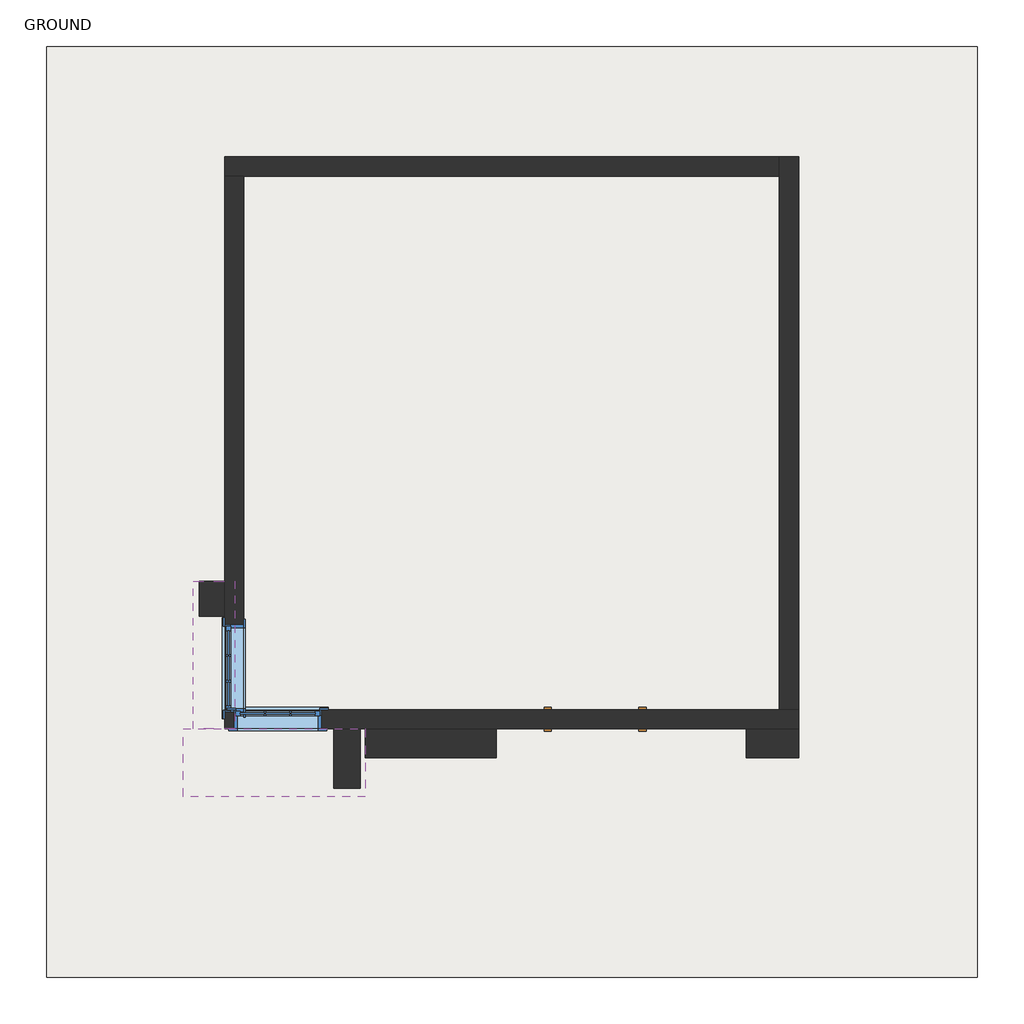
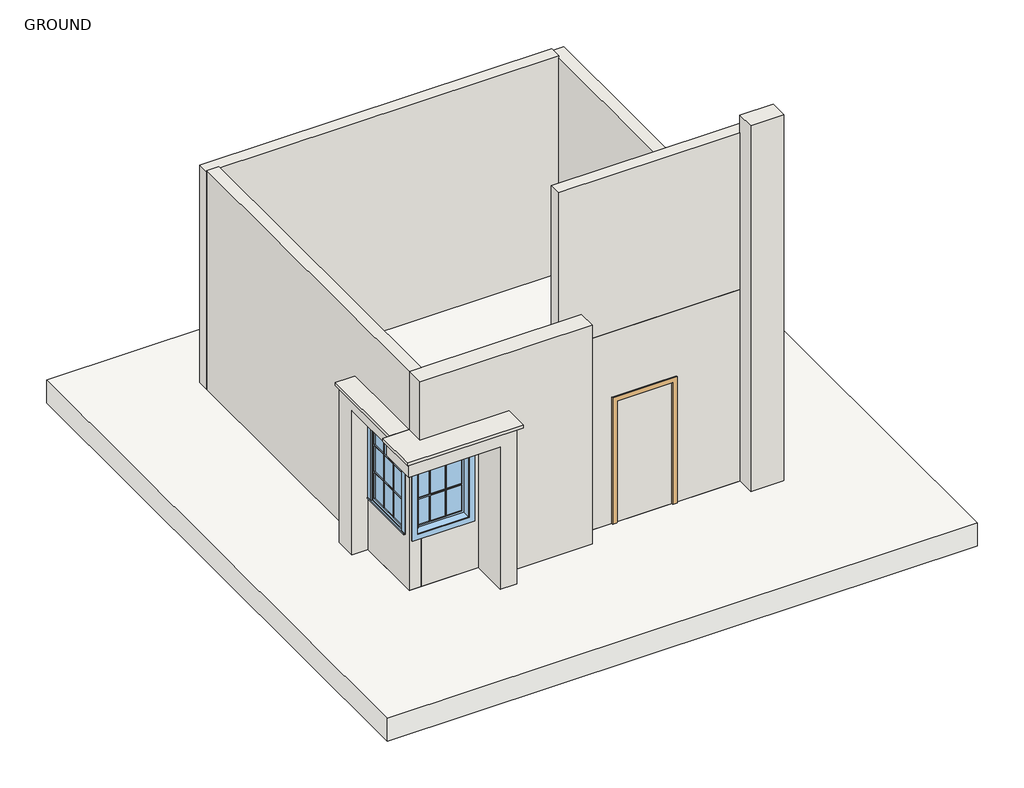
# One storey: 11 walls, 2 slabs, 2 windows, 1 door.
"""IFC4 building model written with IfcOpenShell, lengths in millimetres."""

from ifc_helpers import new_model, si_unit, frame, origin, place, context, project, spatial, polyline, outline, extrude, faceted_brep, transform, mapped, element, save
from components import m_single_flush_0915_x_2134mm_6a9e8738, walls_1_walls_1_8bdf3cb7, walls_10_walls_10_64d1ab67, walls_2_walls_2_b5bda089, walls_3_walls_3_8b246382, walls_5_walls_5_8fe41d8f, walls_6_walls_6_d361cd03, walls_9_walls_9_f00b2fad, window_3d3a5413

model = new_model("IFC4")

# Units and contexts
model_context = context("Model", 3, world=origin())
ifc_project = project(units=[si_unit("LENGTHUNIT", "METRE", prefix="MILLI")], contexts=[model_context])

# Site, building, storey
site = spatial("IfcSite", under=ifc_project)
building = spatial("IfcBuilding", under=site)
storey = spatial("IfcBuildingStorey", under=building, Name="GROUND", Elevation=0.0)

# Door
placement = place(None, origin())
m_single_flush_0915_x_2134mm_shape = m_single_flush_0915_x_2134mm_6a9e8738(model_context)
element("IfcDoor", 1, ObjectType="M_Single-Flush : 0915 x 2134mm", at=placement, inside=storey, context=model_context, shape_type="MappedRepresentation", body=[
    mapped(m_single_flush_0915_x_2134mm_shape, transform((-11916.6283679, -3290.9180898, 0.0), x_axis=(-1.0, 0.0, 0.0), y_axis=(0.0, -1.0, 0.0), z_axis=(0.0, 0.0, 1.0))),
])

# Slabs
element("IfcSlab", 2, ObjectType="Generic Floor - 400mm", at=placement, inside=storey, context=model_context, shape_type="SweptSolid", body=[
    extrude(outline(polyline([(-9784.4289001, -3390.9180898), (-15798.6897324, -3390.9180898), (-15798.6897324, 2600.2819102), (-9784.4289001, 2600.2819102), (-9784.4289001, -3390.9180898)])), frame((0.0, 0.0, -400.0), z_axis=(0.0, 0.0, 1.0), x_axis=(1.0, 0.0, 0.0)), (0.0, 0.0, 1.0), 400.0),
])
element("IfcSlab", 3, ObjectType="Generic Floor - 400mm", at=placement, inside=storey, context=model_context, shape_type="SweptSolid", body=[
    extrude(outline(polyline([(-7910.3714198, 3757.0368614), (-7910.3714198, -5996.5631386), (-17663.9714198, -5996.5631386), (-17663.9714198, 3757.0368614), (-7910.3714198, 3757.0368614)])), frame((0.0, 0.0, -400.0), z_axis=(0.0, 0.0, 1.0), x_axis=(1.0, 0.0, 0.0)), (0.0, 0.0, 1.0), 400.0),
])

# Walls
element("IfcWall", 4, ObjectType="Generic - 9\"", at=placement, inside=storey, context=model_context, shape_type="Brep", body=[
    faceted_brep([(-15798.6897324, 2400.2819102, 0.0), (-15598.6897324, 2400.2819102, 0.0), (-9984.4289001, 2400.2819102, 0.0), (-9984.4289001, 2400.2819102, 3805.8986036), (-15798.6897324, 2400.2819102, 3805.8986036), (-15798.6897324, 2600.2819102, 0.0), (-15798.6897324, 2600.2819102, 3805.8986036), (-9984.4289001, 2600.2819102, 3805.8986036), (-9984.4289001, 2600.2819102, 3774.1343037), (-9984.4289001, 2600.2819102, 0.0)], [[[0, 1, 2, 3, 4]], [[5, 6, 7, 8, 9]], [[2, 1, 0, 5, 9]], [[4, 3, 7, 6]], [[0, 4, 6, 5]], [[3, 2, 9, 8, 7]]]),
])
element("IfcWall", 5, ObjectType="Generic - 9\"", at=placement, inside=storey, context=model_context, shape_type="Brep", body=[
    faceted_brep([(-15598.6897324, -3390.9180898, 0.0), (-15598.6897324, -3190.9180898, 0.0), (-15598.6897324, 2400.2819102, 0.0), (-15598.6897324, 2400.2819102, 3830.5245478), (-15598.6897324, -3390.9180898, 3830.5245478), (-15598.6897324, -3390.9180898, 3352.8), (-15598.6897324, -3390.9180898, 2438.4), (-15598.6897324, -3190.9180898, 2438.4), (-15598.6897324, -2300.3180898, 2438.4), (-15598.6897324, -2300.3180898, 914.4), (-15598.6897324, -3190.9180898, 914.4), (-15598.6897324, -3390.9180898, 914.4), (-15798.6897324, 2400.2819102, 0.0), (-15798.6897324, -3390.9180898, 0.0), (-15798.6897324, -3390.9180898, 3830.5245478), (-15798.6897324, 2400.2819102, 3830.5245478), (-15798.6897324, 2400.2819102, 3805.8986036), (-15798.6897324, -2300.3180898, 914.4), (-15798.6897324, -2300.3180898, 2438.4), (-15798.6897324, -3214.7180898, 2438.4), (-15798.6897324, -3214.7180898, 914.4), (-15698.6897324, -3390.9180898, 914.4), (-15698.6897324, -3390.9180898, 2438.4), (-15698.6897324, -3214.7180898, 914.4), (-15698.6897324, -3214.7180898, 2438.4)], [[[0, 1, 2, 3, 4, 5, 6, 7, 8, 9, 10, 11]], [[12, 13, 14, 15, 16], [17, 18, 19, 20]], [[2, 1, 0, 13, 12]], [[4, 3, 15, 14]], [[4, 14, 13, 0, 11, 21, 22, 6, 5]], [[3, 2, 12, 16, 15]], [[9, 8, 18, 17]], [[17, 20, 23, 21, 11, 10, 9]], [[20, 19, 24, 23]], [[19, 18, 8, 7, 6, 22, 24]], [[21, 23, 24, 22]]]),
])
element("IfcWall", 6, ObjectType="Generic - 9\"", at=placement, inside=storey, context=model_context, shape_type="Brep", body=[
    faceted_brep([(-9784.4289001, -3190.9180898, 0.0), (-9984.4289001, -3190.9180898, 0.0), (-15598.6897324, -3190.9180898, 0.0), (-15598.6897324, -3190.9180898, 914.4), (-14784.2897324, -3190.9180898, 914.4), (-14784.2897324, -3190.9180898, 2438.4), (-15598.6897324, -3190.9180898, 2438.4), (-15598.6897324, -3190.9180898, 3352.8), (-9984.4289001, -3190.9180898, 3352.8), (-9784.4289001, -3190.9180898, 3352.8), (-15598.6897324, -3390.9180898, 0.0), (-9784.4289001, -3390.9180898, 0.0), (-9784.4289001, -3390.9180898, 3352.8), (-9984.4289001, -3390.9180898, 3352.8), (-15598.6897324, -3390.9180898, 3352.8), (-15598.6897324, -3390.9180898, 2438.4), (-14784.2897324, -3390.9180898, 2438.4), (-14784.2897324, -3390.9180898, 914.4), (-15598.6897324, -3390.9180898, 914.4)], [[[0, 1, 2, 3, 4, 5, 6, 7, 8, 9]], [[10, 11, 12, 13, 14, 15, 16, 17, 18]], [[2, 1, 0, 11, 10]], [[9, 8, 7, 14, 13, 12]], [[14, 7, 6, 15]], [[2, 10, 18, 3]], [[16, 5, 4, 17]], [[17, 4, 3, 18]], [[5, 16, 15, 6]], [[9, 12, 11, 0]]]),
])
element("IfcWall", 7, ObjectType="Generic - 9\"", at=placement, inside=storey, context=model_context, shape_type="Brep", body=[
    faceted_brep([(-9984.4289001, 2600.2819102, 0.0), (-9984.4289001, 2400.2819102, 0.0), (-9984.4289001, -3190.9180898, 0.0), (-9984.4289001, -3190.9180898, 3352.8), (-9984.4289001, -3390.9180898, 3352.8), (-9984.4289001, -3390.9180898, 3774.1343037), (-9984.4289001, -3190.9180898, 3774.1343037), (-9984.4289001, 2600.2819102, 3774.1343037), (-9784.4289001, 2600.2819102, 0.0), (-9784.4289001, 2600.2819102, 3774.1343037), (-9784.4289001, -3190.9180898, 3774.1343037), (-9784.4289001, -3390.9180898, 3774.1343037), (-9784.4289001, -3390.9180898, 3352.8), (-9784.4289001, -3190.9180898, 3352.8), (-9784.4289001, -3190.9180898, 0.0)], [[[0, 1, 2, 3, 4, 5, 6, 7]], [[8, 9, 10, 11, 12, 13, 14]], [[2, 1, 0, 8, 14]], [[7, 6, 5, 11, 10, 9]], [[0, 7, 9, 8]], [[12, 4, 3, 13]], [[2, 14, 13, 3]], [[5, 4, 12, 11]]]),
])
walls_1_walls_1_shape = walls_1_walls_1_8bdf3cb7(model_context)
element("IfcWall", 8, ObjectType="Walls 1 : Walls 1", at=placement, inside=storey, context=model_context, shape_type="MappedRepresentation", body=[
    mapped(walls_1_walls_1_shape, transform((0.0, 0.0, 0.0), x_axis=(1.0, 0.0, 0.0), y_axis=(0.0, 1.0, 0.0), z_axis=(0.0, 0.0, 1.0))),
])
walls_10_walls_10_shape = walls_10_walls_10_64d1ab67(model_context)
element("IfcWall", 9, ObjectType="Walls 10 : Walls 10", at=placement, inside=storey, context=model_context, shape_type="MappedRepresentation", body=[
    mapped(walls_10_walls_10_shape, transform((0.0, 0.0, 0.0), x_axis=(1.0, 0.0, 0.0), y_axis=(0.0, 1.0, 0.0), z_axis=(0.0, 0.0, 1.0))),
])
walls_2_walls_2_shape = walls_2_walls_2_b5bda089(model_context)
element("IfcWall", 10, ObjectType="Walls 2 : Walls 2", at=placement, inside=storey, context=model_context, shape_type="MappedRepresentation", body=[
    mapped(walls_2_walls_2_shape, transform((0.0, 0.0, 0.0), x_axis=(1.0, 0.0, 0.0), y_axis=(0.0, 1.0, 0.0), z_axis=(0.0, 0.0, 1.0))),
])
walls_3_walls_3_shape = walls_3_walls_3_8b246382(model_context)
element("IfcWall", 11, ObjectType="Walls 3 : Walls 3", at=placement, inside=storey, context=model_context, shape_type="MappedRepresentation", body=[
    mapped(walls_3_walls_3_shape, transform((0.0, 0.0, 0.0), x_axis=(1.0, 0.0, 0.0), y_axis=(0.0, 1.0, 0.0), z_axis=(0.0, 0.0, 1.0))),
])
walls_5_walls_5_shape = walls_5_walls_5_8fe41d8f(model_context)
element("IfcWall", 12, ObjectType="Walls 5 : Walls 5", at=placement, inside=storey, context=model_context, shape_type="MappedRepresentation", body=[
    mapped(walls_5_walls_5_shape, transform((0.0, 0.0, 0.0), x_axis=(1.0, 0.0, 0.0), y_axis=(0.0, 1.0, 0.0), z_axis=(0.0, 0.0, 1.0))),
])
walls_6_walls_6_shape = walls_6_walls_6_d361cd03(model_context)
element("IfcWall", 13, ObjectType="Walls 6 : Walls 6", at=placement, inside=storey, context=model_context, shape_type="MappedRepresentation", body=[
    mapped(walls_6_walls_6_shape, transform((0.0, 0.0, 0.0), x_axis=(1.0, 0.0, 0.0), y_axis=(0.0, 1.0, 0.0), z_axis=(0.0, 0.0, 1.0))),
])
walls_9_walls_9_shape = walls_9_walls_9_f00b2fad(model_context)
element("IfcWall", 14, ObjectType="Walls 9 : Walls 9", at=placement, inside=storey, context=model_context, shape_type="MappedRepresentation", body=[
    mapped(walls_9_walls_9_shape, transform((0.0, 0.0, 0.0), x_axis=(1.0, 0.0, 0.0), y_axis=(0.0, 1.0, 0.0), z_axis=(0.0, 0.0, 1.0))),
])

# Windows
window_shape = window_3d3a5413(model_context)
element("IfcWindow", 15, ObjectType="Casement 3x3 with Trim : 36\" x 60\"", at=placement, inside=storey, context=model_context, shape_type="MappedRepresentation", body=[
    mapped(window_shape, transform((-15241.4897324, -3290.9180898, 304.8), x_axis=(1.0, 0.0, 0.0), y_axis=(0.0, 1.0, 0.0), z_axis=(0.0, 0.0, 1.0))),
])
element("IfcWindow", 16, ObjectType="Casement 3x3 with Trim : 36\" x 60\"", at=placement, inside=storey, context=model_context, shape_type="MappedRepresentation", body=[
    mapped(window_shape, transform((-15698.6897324, -2757.5180898, 304.8), x_axis=(0.0, 1.0, 0.0), y_axis=(-1.0, 0.0, 0.0), z_axis=(0.0, 0.0, 1.0))),
])

save(model, "model.ifc")

# Revit data of these elements
# Type "M_Single-Flush : 0915 x 2134mm"
#   Type Mark = "15"
#   Thickness = 0' - 2.00787"
#   Height = 7' - 0.01575"
#   Trim Projection Ext = 0' - 0.98425"
#   Trim Projection Int = 0' - 0.98425"
#   Trim Width = 0' - 2.99213"
#   Width = 3' - 0.02362"
#   Door Material = Door - Panel
#   Frame Material = Door - Frame
#   Function = (empty or 0)
#   Wall Closure = (empty or 0)
# Type "Generic Floor - 400mm"
#   Function = 0
#   Layers, outside or top first: 1' - 3.74803" no material (function 1)
# Type "Generic - 9\""
#   Layers, outside or top first: 0' - 7.87402" no material (function 1)
# Type "Casement 3x3 with Trim : 36\" x 60\""
#   Type Mark = "29"
#   Construction Type Id = "GSP4R"
#   Assembly Code = "B2020100"
#   Analytic Construction = "1/8 in Pilkington single glazing"
#   Visual Light Transmittance = 0.9
#   Solar Heat Gain Coefficient = 0.78
#   Heat Transfer Coefficient (U) = 3.6886 W/(m²·K)
#   Height = 5' - 0"
#   Default Sill Height = 2' - 0"
#   Trim Projection - Ext. = 0' - 0 1/2"
#   Trim Projection - Int. = 0' - 0 3/4"
#   Trim Width - Exterior = 0' - 3 1/2"
#   Trim Width - Interior = 0' - 3 1/2"
#   Width = 3' - 0"
#   Window Inset = 0' - 0 3/4"
#   Define Thermal Properties by = 1
#   Glass Pane Material = Glass
#   Sash Material = Sash
#   Trim Exterior Material = Trim
#   Trim Interior Material = Trim
#   Wall Closure = (empty or 0)
# Element 1 (IfcDoor, "M_Single-Flush : 0915 x 2134mm")
#   Phase Created = New Construction
#   Materials on its faces: "Door - Frame", "Door - Panel"
# Elements 2, 3 (IfcSlab, "Generic Floor - 400mm")
#   Height Offset From Level = 0' - 0"
#   Phase Created = New Construction
#   Materials on its faces: "Default Roof"
# Element 4 (IfcWall, "Generic - 9\"")
#   Top Offset = 0' - 0"
#   Base Offset = 0' - 0"
#   Unconnected Height = 12' - 5.83853"
#   wall height = 12' - 5.83853"
#   Phase Created = New Construction
#   Base Constraint = GROUND
#   Materials on its faces: "Default Wall"
# Element 5 (IfcWall, "Generic - 9\"")
#   Top Offset = 0' - 0"
#   Base Offset = 0' - 0"
#   Unconnected Height = 12' - 6.80805"
#   wall height = 12' - 6.80805"
#   Phase Created = New Construction
#   Base Constraint = GROUND
#   Materials on its faces: "Default Wall", "Cherry"
# Element 6 (IfcWall, "Generic - 9\"")
#   Top Offset = 0' - 0"
#   Base Offset = 0' - 0"
#   Unconnected Height = 11' - 0"
#   wall height = 11' - 0"
#   Phase Created = New Construction
#   Base Constraint = GROUND
#   Materials on its faces: "Default Wall", "Cherry"
# Element 7 (IfcWall, "Generic - 9\"")
#   Top Offset = 0' - 0"
#   Base Offset = 0' - 0"
#   Unconnected Height = 12' - 4.58796"
#   wall height = 12' - 4.58796"
#   Phase Created = New Construction
#   Base Constraint = GROUND
#   Materials on its faces: "Default Wall", "Cherry"
# Element 8 (IfcWall, "Walls 1 : Walls 1")
#   Phase Created = New Construction
#   Materials on its faces: "Default Wall"
# Element 9 (IfcWall, "Walls 10 : Walls 10")
#   Phase Created = New Construction
#   Materials on its faces: "Default Wall"
# Element 10 (IfcWall, "Walls 2 : Walls 2")
#   Phase Created = New Construction
#   Materials on its faces: "Default Wall"
# Element 11 (IfcWall, "Walls 3 : Walls 3")
#   Phase Created = New Construction
#   Materials on its faces: "Default Wall"
# Element 12 (IfcWall, "Walls 5 : Walls 5")
#   Phase Created = New Construction
#   Materials on its faces: "Default Wall"
# Element 13 (IfcWall, "Walls 6 : Walls 6")
#   Phase Created = New Construction
#   Materials on its faces: "Default Wall"
# Element 14 (IfcWall, "Walls 9 : Walls 9")
#   Phase Created = New Construction
#   Materials on its faces: "Default Wall"
# Element 15 (IfcWindow, "Casement 3x3 with Trim : 36\" x 60\"")
#   Mark = "6"
#   Phase Created = New Construction
#   Materials on its faces: "Sash", "Glass", "Trim"
# Element 16 (IfcWindow, "Casement 3x3 with Trim : 36\" x 60\"")
#   Mark = "7"
#   Phase Created = New Construction
#   Materials on its faces: "Sash", "Glass", "Trim"
# Materials
#   "Door - Panel": class "Wood", colour RGB 114 82 51, transparency 0
#   "Door - Frame": colour RGB 153 76 43, transparency 0
#   "Glass": class "Glass", colour RGB 218 227 224, transparency 0.85, Description = "Soda Lime Glass", Cost = 0
#   "Sash": class "Wood", colour RGB 136 99 55, transparency 0
#   "Trim": class "Wood", colour RGB 224 178 126, transparency 0
#   "Default Roof": colour RGB 80 80 80, transparency 0
#   "Default Wall": colour RGB 80 80 80, transparency 0
#   "Cherry": class "Wood", colour RGB 154 107 61, transparency 0, Description = "Prunus Serotina", Cost = 0
